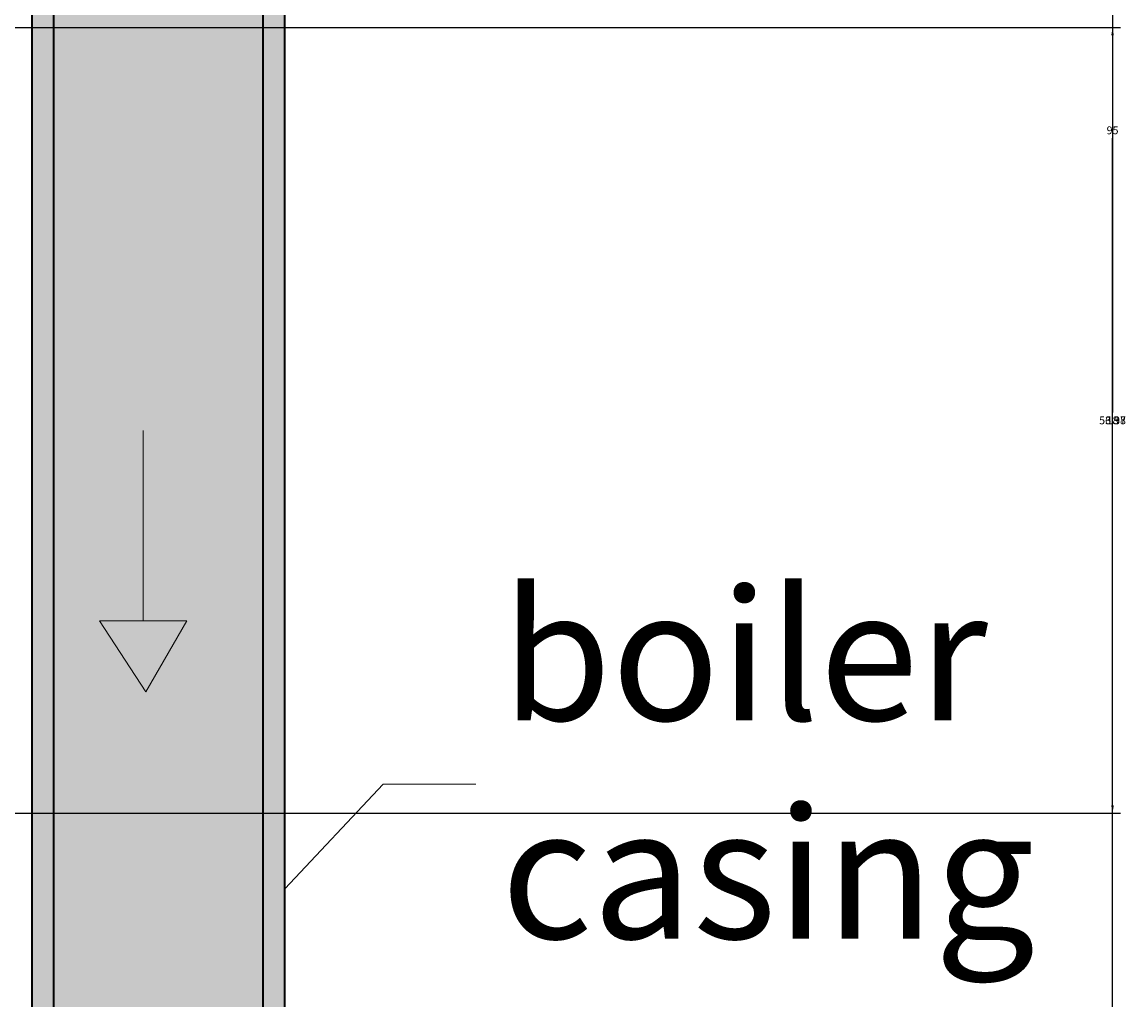
# Model space of a CAD drawing. Units: inches. Extents: x -1 to 292, y -3 to 199.
# Tile 49 of 52: x 267 to 292, y 58 to 81. Entities that reach past the tile are written whole.
import ezdxf

# ---------------------------------------------------------------- set-up
doc = ezdxf.new("R2010")
doc.units = ezdxf.units.IN
doc.header["$MEASUREMENT"] = 0
for name, color, linetype, lineweight in [('M-ANNO-LEAD', 2, 'Continuous', 18), ('M-ANNO-SYMB', 1, 'Continuous', 18), ('M-ANNO-TEXT', 3, 'Continuous', 25), ('M-DIMS', 2, 'Continuous', 18), ('M-EQPM', 7, 'Continuous', 35), ('M-PATT', 8, 'Continuous', 13)]:
    doc.layers.add(name, color=color, linetype=linetype, lineweight=lineweight)
doc.styles.get("Standard").update_dxf_attribs({"font": 'arial.ttf'})
doc.dimstyles.get("Standard").update_dxf_attribs({"dimtxt": 0.18, "dimasz": 0.18, "dimexe": 0.18, "dimexo": 0.0625, "dimgap": 0.09, "dimtad": 0, "dimtih": 1, "dimtoh": 1, "dimdec": 4, "dimzin": 0, "dimdsep": 46, "dimtxsty": 'Standard', "dimcen": 0.09, "dimadec": 0, "dimazin": 0, "dimtfac": 1, "dimtdec": 4, "dimtofl": 0, "dimtmove": 0, "dimatfit": 3, "dimfxl": 1, "dimtolj": 1, "dimtzin": 0, "dimarcsym": 0})

# ---------------------------------------------------------------- blocks, each defined once
blk = doc.blocks.new('FLOW-ARROW-WATER')
blk.add_line((223.29, 53.741), (227.063, 51.564))
blk.add_lwpolyline([(222.79, 52.875), (221.849, 54.506), (223.79, 54.608)], close=True)
blk = doc.blocks.new('*D10')
at = {"layer": 'Defpoints', "color": 0, "transparency": 16777216}
for p in [(169.176, 99.774), (169.176, 43.391), (292.04, 43.391)]:
    blk.add_point(p, dxfattribs=at)
at = {"layer": 'M-DIMS', "color": 0, "lineweight": -2, "transparency": 16777216}
for p, q in [((169.239, 99.774), (292.22, 99.774)), ((292.04, 99.594), (292.04, 71.764)), ((292.04, 43.571), (292.04, 71.4)), ((169.239, 43.391), (292.22, 43.391))]:
    blk.add_line(p, q, dxfattribs=at)
at = {"layer": 'M-DIMS', "color": 0, "transparency": 16777216}
for points in [[(292.01, 99.594), (292.07, 99.594), (292.04, 99.774)], [(292.01, 43.571), (292.07, 43.571), (292.04, 43.391)]]:
    blk.add_solid(points, dxfattribs=at)
at = {"layer": 'M-DIMS', "color": 0, "transparency": 16777216, "insert": (292.04, 71.582), "char_height": 0.18, "attachment_point": 5}
blk.add_mtext('\\A1;56.38', dxfattribs=at)
blk = doc.blocks.new('*D25')
at = {"layer": 'Defpoints', "color": 0, "transparency": 16777216}
for p in [(273.066, 88.419), (215.241, 88.13), (273.066, -2.71)]:
    blk.add_point(p, dxfattribs=at)
at = {"layer": 'M-DIMS', "color": 0, "lineweight": -2, "transparency": 16777216}
for p, q in [((273.066, 88.357), (273.066, -2.89)), ((215.241, 88.068), (215.241, -2.89)), ((215.421, -2.71), (243.76, -2.71)), ((272.886, -2.71), (244.547, -2.71))]:
    blk.add_line(p, q, dxfattribs=at)
at = {"layer": 'M-DIMS', "color": 0, "transparency": 16777216}
for points in [[(215.421, -2.68), (215.421, -2.74), (215.241, -2.71)], [(272.886, -2.68), (272.886, -2.74), (273.066, -2.71)]]:
    blk.add_solid(points, dxfattribs=at)
at = {"layer": 'M-DIMS', "color": 0, "transparency": 16777216, "insert": (244.153, -2.71), "char_height": 0.18, "attachment_point": 5}
blk.add_mtext('\\A1;57.83', dxfattribs=at)
blk = doc.blocks.new('*D29')
at = {"layer": 'Defpoints', "color": 0, "transparency": 16777216}
for p in [(243.903, 98.567), (243.903, 44.598), (292.04, 44.598)]:
    blk.add_point(p, dxfattribs=at)
at = {"layer": 'M-DIMS', "color": 0, "lineweight": -2, "transparency": 16777216}
for p, q in [((243.966, 98.567), (292.22, 98.567)), ((292.04, 98.387), (292.04, 71.764)), ((292.04, 44.778), (292.04, 71.4)), ((243.966, 44.598), (292.22, 44.598))]:
    blk.add_line(p, q, dxfattribs=at)
at = {"layer": 'M-DIMS', "color": 0, "transparency": 16777216}
for points in [[(292.01, 98.387), (292.07, 98.387), (292.04, 98.567)], [(292.01, 44.778), (292.07, 44.778), (292.04, 44.598)]]:
    blk.add_solid(points, dxfattribs=at)
at = {"layer": 'M-DIMS', "color": 0, "transparency": 16777216, "insert": (292.04, 71.582), "char_height": 0.18, "attachment_point": 5}
blk.add_mtext('\\A1;53.97', dxfattribs=at)
blk = doc.blocks.new('*D31')
at = {"layer": 'Defpoints', "color": 0, "transparency": 16777216}
for p in [(254.903, 80.582), (292.04, 80.582), (254.903, 62.582)]:
    blk.add_point(p, dxfattribs=at)
at = {"layer": 'M-DIMS', "color": 0, "lineweight": -2, "transparency": 16777216}
for p, q in [((254.966, 80.582), (292.22, 80.582)), ((292.04, 80.402), (292.04, 71.764)), ((292.04, 62.762), (292.04, 71.4)), ((254.966, 62.582), (292.22, 62.582))]:
    blk.add_line(p, q, dxfattribs=at)
at = {"layer": 'M-DIMS', "color": 0, "transparency": 16777216}
for points in [[(292.01, 80.402), (292.07, 80.402), (292.04, 80.582)], [(292.01, 62.762), (292.07, 62.762), (292.04, 62.582)]]:
    blk.add_solid(points, dxfattribs=at)
at = {"layer": 'M-DIMS', "color": 0, "transparency": 16777216, "insert": (292.04, 71.582), "char_height": 0.18, "attachment_point": 5}
blk.add_mtext('\\A1;18', dxfattribs=at)
blk = doc.blocks.new('*D33')
at = {"layer": 'Defpoints', "color": 0, "transparency": 16777216}
for p in [(242.955, 125.727), (292.04, 125.727), (237.933, 30.73)]:
    blk.add_point(p, dxfattribs=at)
at = {"layer": 'M-DIMS', "color": 0, "lineweight": -2, "transparency": 16777216}
for p, q in [((243.018, 125.727), (292.22, 125.727)), ((292.04, 125.547), (292.04, 78.41)), ((292.04, 30.91), (292.04, 78.046)), ((237.996, 30.73), (292.22, 30.73))]:
    blk.add_line(p, q, dxfattribs=at)
at = {"layer": 'M-DIMS', "color": 0, "transparency": 16777216}
for points in [[(292.01, 125.547), (292.07, 125.547), (292.04, 125.727)], [(292.01, 30.91), (292.07, 30.91), (292.04, 30.73)]]:
    blk.add_solid(points, dxfattribs=at)
at = {"layer": 'M-DIMS', "color": 0, "transparency": 16777216, "insert": (292.04, 78.228), "char_height": 0.18, "attachment_point": 5}
blk.add_mtext('\\A1;95', dxfattribs=at)

msp = doc.modelspace()

# ---------------------------------------------------------------- hatches: boundary and pattern name
at = {"layer": 'M-PATT'}
h = msp.add_hatch(color=256, dxfattribs=at)
h.set_gradient(color1=(0, 255, 255), color2=(0, 255, 255), tint=1, name='CYLINDER')
h.paths.add_polyline_path([(256.8092, 99.5764), (256.4077, 99.3157), (253.7155, 100.87), (251.3221, 99.3157), (248.6299, 100.87), (246.2365, 99.3157), (243.5443, 100.87), (241.1509, 99.3157), (238.4587, 100.87), (236.4209, 99.5466), (236.4209, 97.1861), (234.9209, 97.1861), (234.9209, 99.9764), (233.3731, 100.87), (230.9797, 99.3157, 1.0704128)])
h.paths.add_polyline_path([(234.4549, 44.5975, 1), (253.3518, 44.5975, 1)])
h.paths.add_polyline_path([(235.4822, 48.8821), (220.034, 57.8011), (220.034, 85.363), (232.4507, 92.5318, -0.0853739), (231.0925, 96.7051), (215.7407, 87.8418), (215.7407, 55.3224), (234.4552, 44.5176, -0.0021162), (234.4549, 44.5975, -0.1182098)])
h.paths.add_polyline_path([(222.7904, 52.8755), (221.8492, 54.5058), (223.7904, 54.6075)], flags=16)
h.paths.add_polyline_path([(216.828, 66.8912), (217.7692, 68.5216), (218.828, 66.8912)], flags=16)
h.paths.add_polyline_path([(216.8084, 83.826), (217.7497, 85.4564), (218.8084, 83.826)], flags=16)
h.paths.add_polyline_path([(226.468, 92.8803), (228.3442, 93.0348), (227.6068, 91.2362)], flags=16)
h.paths.add_polyline_path([(272.5659, 88.1304), (260.2765, 95.2257), (259.0113, 93.0196), (263.0639, 91.1046), (263.4912, 92.0087), (264.5631, 90.4612), (262.6367, 90.2004), (263.0639, 91.1046), (259.0113, 93.0196), (257.8918, 91.0677), (267.7726, 85.363), (267.7726, 57.8011), (255.5043, 50.718), (257.0663, 46.085), (272.5659, 55.0337)])
h.paths.add_polyline_path([(263.6286, 51.5636), (261.7461, 51.5636), (262.6286, 53.2956)], flags=16)
h.paths.add_polyline_path([(269.8773, 65.3608), (268.8186, 66.9911), (270.8186, 66.9911)], flags=16)
h.paths.add_polyline_path([(269.8773, 80.8843), (268.8186, 82.5146), (270.8186, 82.5146)], flags=16)
h.paths.add_polyline_path([(255.5043, 50.718), (252.3244, 48.8821, -0.1182098), (253.3518, 44.5975, -0.0177685), (253.3279, 43.9266), (257.0663, 46.085)])
h.paths.add_polyline_path([(260.2765, 95.2257), (256.7809, 97.2439, -0.0959457), (255.356, 92.5318), (257.8918, 91.0677)])
h = msp.add_hatch(color=256, dxfattribs=at)
h.set_gradient(color1=(76, 38, 47), color2=(76, 38, 47), tint=1, name='CYLINDER')
h.paths.add_polyline_path([(267.2726, 58.0898), (255.3414, 51.2013), (255.5043, 50.718), (267.7726, 57.8011), (267.7726, 85.363), (257.8918, 91.0677), (257.643, 90.634), (267.2726, 85.0743)])
h.paths.add_polyline_path([(272.5659, 55.0337), (257.0663, 46.085), (257.2293, 45.6017), (273.0659, 54.745), (273.0659, 88.4191), (260.5253, 95.6595), (260.2765, 95.2257), (272.5659, 88.1304)])
h.paths.add_polyline_path([(215.2407, 55.0337), (234.4787, 43.9266, -0.0156517), (234.4552, 44.5176), (215.7407, 55.3224), (215.7407, 87.8418), (231.0925, 96.7051, -0.0104859), (231.0257, 97.2439), (215.2407, 88.1304)])
h.paths.add_polyline_path([(220.034, 57.8011), (235.4822, 48.8821, -0.0132367), (235.7207, 49.3218), (220.534, 58.0898), (220.534, 85.0743), (232.6923, 92.0939, -0.0096587), (232.4507, 92.5318), (220.034, 85.363)])
h = msp.add_hatch(color=256, dxfattribs=at)
h.set_gradient(color1=(0, 0, 255), color2=(0, 0, 255), tint=1, name='CYLINDER')
h.paths.add_polyline_path([(227.6068, 91.2362), (228.3442, 93.0348), (226.468, 92.8803)])
h.paths.add_polyline_path([(218.8084, 83.826), (217.7497, 85.4564), (216.8084, 83.826)])
h.paths.add_polyline_path([(262.6367, 90.2004), (264.5631, 90.4612), (263.4912, 92.0087)])
h.paths.add_polyline_path([(217.7692, 68.5216), (216.828, 66.8912), (218.828, 66.8912)])
h.paths.add_polyline_path([(223.7904, 54.6075), (221.8492, 54.5058), (222.7904, 52.8755)])
h.paths.add_polyline_path([(262.6286, 53.2956), (261.7461, 51.5636), (263.6286, 51.5636)])
h.paths.add_polyline_path([(268.8186, 82.5146), (269.8773, 80.8843), (270.8186, 82.5146)])
h.paths.add_polyline_path([(268.8186, 66.9911), (269.8773, 65.3608), (270.8186, 66.9911)])

# ---------------------------------------------------------------- linework, layer by layer
at = {"layer": 'M-ANNO-LEAD'}
for p, q in [((273.0659, 60.8492), (275.3157, 63.2444)), ((275.3157, 63.2444), (277.4399, 63.2444))]:
    msp.add_line(p, q, dxfattribs=at)
at = {"layer": 'M-EQPM'}
for points in [[(253.2639, 43.3124), (273.0659, 54.745), (273.0659, 88.4191), (256.8257, 97.7954)], [(253.3279, 43.9266), (272.5659, 55.0337), (272.5659, 88.1304), (256.7809, 97.2439)], [(252.3359, 48.8887), (267.7726, 57.8011), (267.7726, 85.363), (255.356, 92.5318)], [(252.0859, 49.3218), (267.2726, 58.0898), (267.2726, 85.0743), (255.1143, 92.0939)]]:
    msp.add_lwpolyline(points, dxfattribs=at)

# ---------------------------------------------------------------- block references
at = {"layer": 'M-ANNO-SYMB', "rotation": 120.0000000000007}
msp.add_blockref('FLOW-ARROW-WATER', (428.0053, -99.5133), dxfattribs=at)

# ---------------------------------------------------------------- texts
at = {"layer": 'M-ANNO-TEXT', "insert": (278.0232, 67.7073), "char_height": 3, "attachment_point": 1}
msp.add_mtext_dynamic_manual_height_columns('boiler\\Pcasing', width=23.906137, gutter_width=1, heights=[0], dxfattribs=at)

# ---------------------------------------------------------------- dimensions: what is measured, and where the dimension line sits
at = {"layer": 'M-DIMS'}
for base, p1, p2, override, picture, middle in [((292.0399, 125.7269), (237.9333, 30.7296), (242.9552, 125.7269), {"dimdec": 0, "dimlfac": 1, "dimrnd": 0, "dimzin": 0, "dimdsep": 46, "dimlunit": 2}, '*D33', (292.0399, 78.2282)), ((292.0399, 43.3906), (169.176, 99.7735), (169.176, 43.3906), {"dimdec": 2, "dimlfac": 1, "dimrnd": 0, "dimzin": 0, "dimdsep": 46, "dimlunit": 2}, '*D10', (292.0399, 71.5821)), ((292.0399, 44.5975), (243.9033, 98.5666), (243.9033, 44.5975), {"dimdec": 2, "dimlfac": 1, "dimrnd": 0, "dimzin": 0, "dimdsep": 46, "dimlunit": 2}, '*D29', (292.0399, 71.5821)), ((292.0399, 80.5821), (254.9033, 62.5821), (254.9033, 80.5821), {"dimdec": 0, "dimlfac": 1, "dimrnd": 0, "dimzin": 0, "dimdsep": 46, "dimlunit": 2}, '*D31', (292.0399, 71.5821))]:
    dim = msp.add_linear_dim(base=base, p1=p1, p2=p2, angle=90, dimstyle='Standard', override=override, dxfattribs=at)
    dim.commit()
    dim.dimension.update_dxf_attribs({"geometry": picture, "text_midpoint": middle})
dim = msp.add_linear_dim(base=(273.0659, -2.7104), p1=(215.2407, 88.1304), p2=(273.0659, 88.4191), dimstyle='Standard', override={"dimdec": 2, "dimlfac": 1, "dimrnd": 0, "dimzin": 0, "dimdsep": 46, "dimlunit": 2}, dxfattribs=at)
dim.commit()
dim.dimension.update_dxf_attribs({"geometry": '*D25', "text_midpoint": (244.1533, -2.7104)})

doc.saveas('drawing.dxf')
